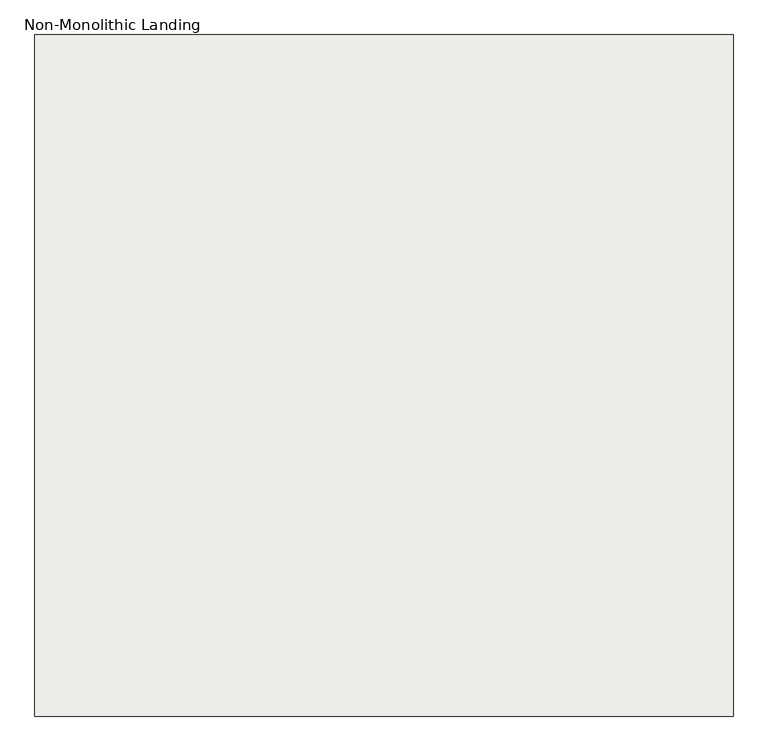
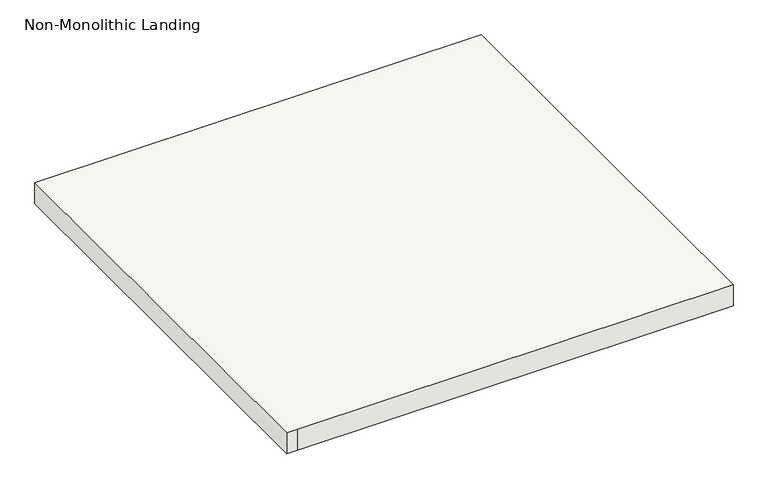
"""IFC4 building model written with IfcOpenShell, lengths in millimetres: slab geometry, Non-Monolithic Landing."""

from ifc_helpers import new_model, si_unit, frame, origin, place, context, project, spatial, polyline, outline, extrude, source, transform, mapped, element, save


def non_monolithic_landing_f8b46ba6(model_context):
    return source(origin(), model_context, "Body", "SweptSolid", [
        extrude(outline(polyline([(-10492.1794909, -1507.9618509), (-9477.5794909, -1507.9618509), (-9477.5794909, -2498.5618509), (-10468.1794909, -2498.5618509), (-10492.1794909, -2498.5618509), (-10492.1794909, -1507.9618509)])), frame((0.0, 0.0, 1267.8117647), z_axis=(0.0, 0.0, 1.0), x_axis=(1.0, 0.0, 0.0)), (0.0, 0.0, 1.0), 50.0),
    ])


if __name__ == "__main__":
    model = new_model("IFC4")
    model_context = context("Model", 3, world=origin())
    ifc_project = project(units=[si_unit("LENGTHUNIT", "METRE", prefix="MILLI")], contexts=[model_context])
    site = spatial("IfcSite", under=ifc_project)
    building = spatial("IfcBuilding", under=site)
    placement = place(None, origin())
    non_monolithic_landing_shape = non_monolithic_landing_f8b46ba6(model_context)
    element("IfcSlab", 1, ObjectType="Non-Monolithic Landing", at=placement, inside=building, context=model_context, shape_type="MappedRepresentation", body=[
        mapped(non_monolithic_landing_shape, transform((0.0, 0.0, 0.0), x_axis=(1.0, 0.0, 0.0), y_axis=(0.0, 1.0, 0.0), z_axis=(0.0, 0.0, 1.0))),
    ])
    save(model, "model.ifc")
